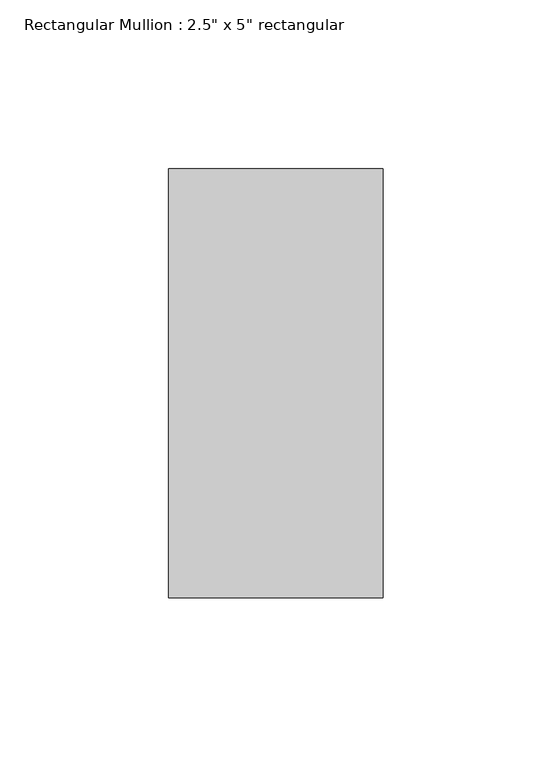
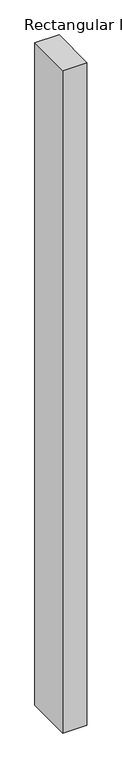
"""IFC4 building model written with IfcOpenShell, lengths in millimetres: member geometry."""

from ifc_helpers import new_model, si_unit, frame, origin, place, context, project, spatial, polyline, outline, extrude, source, transform, mapped, element, save


def member_eeaa0ee0(model_context):
    return source(origin(), model_context, "Body", "SweptSolid", [
        extrude(outline(polyline([(31.75, 63.5), (31.75, -63.5), (-31.75, -63.5), (-31.75, 63.5), (31.75, 63.5)])), frame((0.0, 0.0, -1843.0744962), z_axis=(0.0, 0.0, 1.0), x_axis=(1.0, 0.0, 0.0)), (0.0, 0.0, 1.0), 1843.0744962),
    ])


if __name__ == "__main__":
    model = new_model("IFC4")
    model_context = context("Model", 3, world=origin())
    ifc_project = project(units=[si_unit("LENGTHUNIT", "METRE", prefix="MILLI")], contexts=[model_context])
    site = spatial("IfcSite", under=ifc_project)
    building = spatial("IfcBuilding", under=site)
    placement = place(None, origin())
    member_shape = member_eeaa0ee0(model_context)
    element("IfcMember", 1, ObjectType="Rectangular Mullion : 2.5\" x 5\" rectangular", at=placement, inside=building, context=model_context, shape_type="MappedRepresentation", body=[
        mapped(member_shape, transform((0.0, 0.0, 0.0), x_axis=(1.0, 0.0, 0.0), y_axis=(0.0, 1.0, 0.0), z_axis=(0.0, 0.0, 1.0))),
    ])
    save(model, "model.ifc")

# Revit data of these elements
# Type "Rectangular Mullion : 2.5\" x 5\" rectangular"
#   built-in parameter 1007304 = 0.416667 (stored number, unit not read)
#   built-in parameter 1007301 = 0.104167 (stored number, unit not read)
#   built-in parameter 1007300 = 0.104167 (stored number, unit not read)
# Element 1 (IfcMember, "Rectangular Mullion : 2.5\" x 5\" rectangular")
#   Materials on its faces: "Aluminum"
# Materials
#   "Aluminum": class "Metal", colour RGB 247 247 247, transparency 0, Description = "Aluminum 6061", Cost = 0
